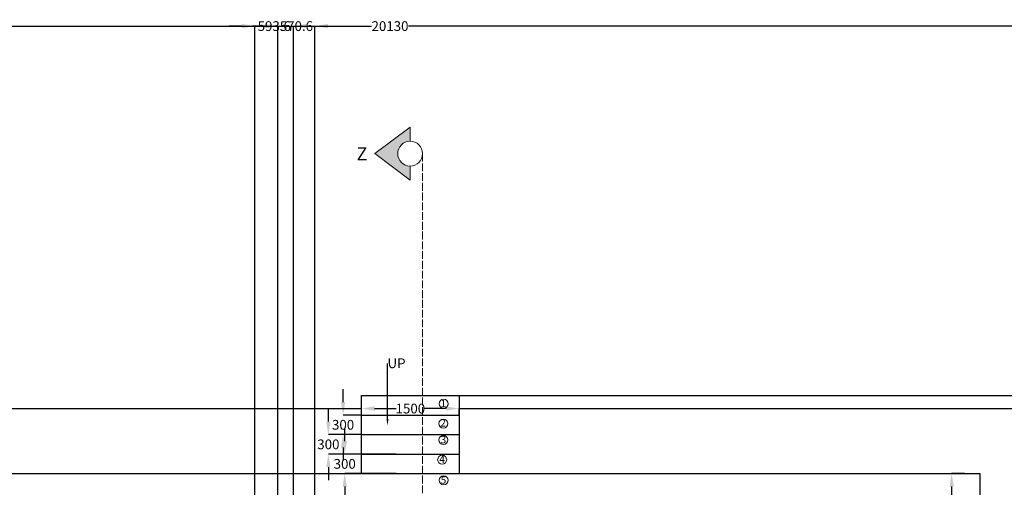
# Model space of a CAD drawing. Units: inches. Extents: x 22626 to 57351, y 2118 to 36234.
# Tile 9 of 10: x 34432 to 49561, y 29046 to 36234. Entities that reach past the tile are written whole.
import ezdxf
from ezdxf import colors
from ezdxf.entities.mleader import LeaderData, LeaderLine
from ezdxf.math import Vec2, Vec3

# ---------------------------------------------------------------- set-up
doc = ezdxf.new("R2010")
doc.units = ezdxf.units.IN
doc.header["$MEASUREMENT"] = 0
doc.linetypes.add('ACAD_ISO02W100', pattern=[15, 12, -3])
for name, color, linetype, lineweight in [('A-ANNO-DIMS', 130, 'Continuous', 18), ('A-ANNO-STRS', 130, 'Continuous', 15), ('A-ANNO-SYMB', 130, 'Continuous', 18), ('A-FLOR', 80, 'Continuous', 30), ('A-ROOF', 80, 'Continuous', 25), ('STAIRS', 82, 'Continuous', 25)]:
    doc.layers.add(name, color=color, linetype=linetype, lineweight=lineweight)
doc.layers.add('A-SECT', color=2, linetype='ACAD_ISO02W100', lineweight=18, true_color=0xf1eb1f)
doc.styles.get("Standard").update_dxf_attribs({"font": 'arial.ttf'})
doc.dimstyles.get("Standard").update_dxf_attribs({"dimtxt": 150, "dimasz": 200, "dimexe": 0.18, "dimexo": 0.0625, "dimgap": 0.09, "dimtad": 0, "dimtih": 1, "dimtoh": 1, "dimdec": 0, "dimzin": 0, "dimdsep": 46, "dimtxsty": 'Standard', "dimcen": 0.09, "dimadec": 0, "dimazin": 0, "dimtfac": 1, "dimtdec": 0, "dimtofl": 0, "dimtmove": 0, "dimatfit": 3, "dimfxl": 1, "dimtolj": 1, "dimtzin": 0, "dimarcsym": 0})

# ---------------------------------------------------------------- blocks, each defined once
blk = doc.blocks.new('*D20')
at = {"layer": 'A-ANNO-DIMS', "color": 0, "lineweight": -2, "transparency": 16777216}
for p, q in [((39426, 29757), (39426, 29957)), ((40218, 29557), (39426, 29557)), ((40218, 29257), (39426, 29257)), ((39426, 29057), (39426, 28857))]:
    blk.add_line(p, q, dxfattribs=at)
at = {"layer": 'A-ANNO-DIMS', "color": 0, "transparency": 16777216}
for points in [[(39393, 29757), (39460, 29757), (39426, 29557)], [(39393, 29057), (39460, 29057), (39426, 29257)]]:
    blk.add_solid(points, dxfattribs=at)
at = {"layer": 'Defpoints', "color": 0, "transparency": 16777216}
for p in [(39426, 29557), (40218, 29557), (40218, 29257)]:
    blk.add_point(p, dxfattribs=at)
at = {"layer": 'A-ANNO-DIMS', "color": 0, "transparency": 16777216, "insert": (39426, 29407), "char_height": 150, "attachment_point": 5}
blk.add_mtext('\\A1;300', dxfattribs=at)
blk = doc.blocks.new('*D21')
at = {"layer": 'A-ANNO-DIMS', "color": 0, "lineweight": -2, "transparency": 16777216}
for p, q in [((39175, 30057), (39175, 30257)), ((39684, 29857), (39175, 29857)), ((39684, 29557), (39175, 29557)), ((39175, 29357), (39175, 29157))]:
    blk.add_line(p, q, dxfattribs=at)
at = {"layer": 'A-ANNO-DIMS', "color": 0, "transparency": 16777216}
for points in [[(39142, 30057), (39208, 30057), (39175, 29857)], [(39142, 29357), (39208, 29357), (39175, 29557)]]:
    blk.add_solid(points, dxfattribs=at)
at = {"layer": 'Defpoints', "color": 0, "transparency": 16777216}
for p in [(39175, 29857), (39685, 29857), (39685, 29557)]:
    blk.add_point(p, dxfattribs=at)
at = {"layer": 'A-ANNO-DIMS', "color": 0, "transparency": 16777216, "insert": (39175, 29707), "char_height": 150, "attachment_point": 5}
blk.add_mtext('\\A1;300', dxfattribs=at)
blk = doc.blocks.new('*D22')
at = {"layer": 'A-ANNO-DIMS', "color": 0, "lineweight": -2, "transparency": 16777216}
for p, q in [((39401, 30357), (39401, 30557)), ((39684, 30157), (39401, 30157)), ((39684, 29857), (39401, 29857)), ((39401, 29657), (39401, 29457))]:
    blk.add_line(p, q, dxfattribs=at)
at = {"layer": 'A-ANNO-DIMS', "color": 0, "transparency": 16777216}
for points in [[(39368, 30357), (39435, 30357), (39401, 30157)], [(39368, 29657), (39435, 29657), (39401, 29857)]]:
    blk.add_solid(points, dxfattribs=at)
at = {"layer": 'Defpoints', "color": 0, "transparency": 16777216}
for p in [(39401, 30157), (39685, 30157), (39685, 29857)]:
    blk.add_point(p, dxfattribs=at)
at = {"layer": 'A-ANNO-DIMS', "color": 0, "transparency": 16777216, "insert": (39401, 30007), "char_height": 150, "attachment_point": 5}
blk.add_mtext('\\A1;300', dxfattribs=at)
blk = doc.blocks.new('*D23')
at = {"layer": 'A-ANNO-DIMS', "color": 0, "lineweight": -2, "transparency": 16777216}
for p, q in [((39685, 30157), (39685, 30257)), ((39885, 30257), (40218, 30257)), ((40985, 30257), (40651, 30257)), ((41185, 30157), (41185, 30257))]:
    blk.add_line(p, q, dxfattribs=at)
at = {"layer": 'A-ANNO-DIMS', "color": 0, "transparency": 16777216}
for points in [[(39885, 30290), (39885, 30224), (39685, 30257)], [(40985, 30290), (40985, 30224), (41185, 30257)]]:
    blk.add_solid(points, dxfattribs=at)
at = {"layer": 'Defpoints', "color": 0, "transparency": 16777216}
for p in [(39685, 30157), (41185, 30257), (41185, 30157)]:
    blk.add_point(p, dxfattribs=at)
at = {"layer": 'A-ANNO-DIMS', "color": 0, "transparency": 16777216, "insert": (40435, 30257), "char_height": 150, "attachment_point": 5}
blk.add_mtext('\\A1;1500', dxfattribs=at)
blk = doc.blocks.new('*D24')
at = {"layer": 'A-ANNO-DIMS', "color": 0, "lineweight": -2, "transparency": 16777216}
for p, q in [((48951, 29257), (48752, 29257)), ((48752, 29057), (48752, 28834)), ((48752, 28457), (48752, 28680)), ((48951, 28257), (48752, 28257))]:
    blk.add_line(p, q, dxfattribs=at)
at = {"layer": 'A-ANNO-DIMS', "color": 0, "transparency": 16777216}
for points in [[(48719, 29057), (48786, 29057), (48752, 29257)], [(48719, 28457), (48786, 28457), (48752, 28257)]]:
    blk.add_solid(points, dxfattribs=at)
at = {"layer": 'Defpoints', "color": 0, "transparency": 16777216}
for p in [(48752, 29257), (48951, 29257), (48951, 28257)]:
    blk.add_point(p, dxfattribs=at)
at = {"layer": 'A-ANNO-DIMS', "color": 0, "transparency": 16777216, "insert": (48752, 28757), "char_height": 150, "attachment_point": 5}
blk.add_mtext('\\A1;1000', dxfattribs=at)
blk = doc.blocks.new('SECTION-HEAD')
h = blk.add_hatch(color=256)
h.dxf.hatch_style = 1
h.paths.add_polyline_path([(815, 541), (599, 541, -1), (216, 541), (0, 541), (407, 0)])
for p, q in [((216, 541), (0, 541)), ((0, 541), (407, 0)), ((815, 541), (407, 0)), ((599, 541), (815, 541))]:
    blk.add_line(p, q)
blk.add_circle((407, 541), 191)
blk = doc.blocks.new('*D98')
at = {"layer": 'A-ANNO-DIMS', "color": 0, "lineweight": -2, "transparency": 16777216}
for p, q in [((30057, 30257), (30057, 36136)), ((30257, 36136), (39839, 36136)), ((49987, 36136), (40406, 36136)), ((50187, 30257), (50187, 36136))]:
    blk.add_line(p, q, dxfattribs=at)
at = {"layer": 'A-ANNO-DIMS', "color": 0, "transparency": 16777216}
for points in [[(30257, 36169), (30257, 36103), (30057, 36136)], [(49987, 36169), (49987, 36103), (50187, 36136)]]:
    blk.add_solid(points, dxfattribs=at)
at = {"layer": 'Defpoints', "color": 0, "transparency": 16777216}
for p in [(50187, 36136), (30057, 30257), (50187, 30257)]:
    blk.add_point(p, dxfattribs=at)
at = {"layer": 'A-ANNO-DIMS', "color": 0, "transparency": 16777216, "insert": (40122, 36136), "char_height": 150, "attachment_point": 5}
blk.add_mtext('\\A1;20130', dxfattribs=at)
blk = doc.blocks.new('*D99')
at = {"layer": 'A-ANNO-DIMS', "color": 0, "lineweight": -2, "transparency": 16777216}
for p, q in [((41185, 30457), (57039, 30457)), ((57039, 30257), (57039, 18934)), ((57039, 7457), (57039, 18780)), ((43702, 7257), (57039, 7257))]:
    blk.add_line(p, q, dxfattribs=at)
at = {"layer": 'A-ANNO-DIMS', "color": 0, "transparency": 16777216}
for points in [[(57005, 30257), (57072, 30257), (57039, 30457)], [(57005, 7457), (57072, 7457), (57039, 7257)]]:
    blk.add_solid(points, dxfattribs=at)
at = {"layer": 'Defpoints', "color": 0, "transparency": 16777216}
for p in [(41185, 30457), (57039, 30457), (43702, 7257)]:
    blk.add_point(p, dxfattribs=at)
at = {"layer": 'A-ANNO-DIMS', "color": 0, "transparency": 16777216, "insert": (57039, 18857), "char_height": 150, "attachment_point": 5}
blk.add_mtext('\\A1;23200', dxfattribs=at)
blk = doc.blocks.new('*D106')
at = {"layer": 'A-ANNO-DIMS', "color": 0, "lineweight": -2, "transparency": 16777216}
for p, q in [((38198, 36136), (37998, 36136)), ((38398, 21952), (38398, 36136)), ((38969, 21952), (38969, 36136)), ((39169, 36136), (39369, 36136))]:
    blk.add_line(p, q, dxfattribs=at)
at = {"layer": 'A-ANNO-DIMS', "color": 0, "transparency": 16777216}
for points in [[(38198, 36169), (38198, 36103), (38398, 36136)], [(39169, 36169), (39169, 36103), (38969, 36136)]]:
    blk.add_solid(points, dxfattribs=at)
at = {"layer": 'Defpoints', "color": 0, "transparency": 16777216}
for p in [(38969, 36136), (38398, 21952), (38969, 21952)]:
    blk.add_point(p, dxfattribs=at)
at = {"layer": 'A-ANNO-DIMS', "color": 0, "transparency": 16777216, "insert": (38684, 36136), "char_height": 150, "attachment_point": 5}
blk.add_mtext('\\A1;570.6', dxfattribs=at)
blk = doc.blocks.new('*D108')
at = {"layer": 'A-ANNO-DIMS', "color": 0, "lineweight": -2, "transparency": 16777216}
for p, q in [((37847, 36136), (37647, 36136)), ((38047, 24856), (38047, 36136)), ((38641, 24856), (38641, 36136)), ((38841, 36136), (39041, 36136))]:
    blk.add_line(p, q, dxfattribs=at)
at = {"layer": 'A-ANNO-DIMS', "color": 0, "transparency": 16777216}
for points in [[(37847, 36169), (37847, 36103), (38047, 36136)], [(38841, 36169), (38841, 36103), (38641, 36136)]]:
    blk.add_solid(points, dxfattribs=at)
at = {"layer": 'Defpoints', "color": 0, "transparency": 16777216}
for p in [(38641, 36136), (38047, 24856), (38641, 24856)]:
    blk.add_point(p, dxfattribs=at)
at = {"layer": 'A-ANNO-DIMS', "color": 0, "transparency": 16777216, "insert": (38344, 36136), "char_height": 150, "attachment_point": 5}
blk.add_mtext('\\A1;593.6', dxfattribs=at)

msp = doc.modelspace()

# ---------------------------------------------------------------- linework, layer by layer
at = {"layer": 'A-ANNO-STRS'}
for centre in [(40946.5, 30330.65), (40940.93, 30026.37), (40943.28, 29775.32), (40923.6, 29469.73), (40946.5, 29155.17)]:
    msp.add_circle(centre, 69.29, dxfattribs=at)
at = {"layer": 'A-FLOR'}
for p, q in [((31057.43, 29256.86), (49187.43, 29256.86)), ((49187.43, 29256.86), (49187.43, 27806.86))]:
    msp.add_line(p, q, dxfattribs=at)
at = {"layer": 'A-ROOF'}
for points in [[(43702.43, 11956.86), (43702.43, 7256.86), (37542.43, 7256.86), (37542.43, 11956.86), (32562.43, 11956.86), (32562.43, 22296.86), (30057.43, 22296.86), (30057.43, 24356.86), (30057.43, 30256.86), (39684.53, 30256.86)], [(41184.53, 30256.86), (50187.43, 30256.86), (50187.43, 25126.86), (50187.43, 22296.86), (48682.43, 22296.86), (48682.43, 11956.86), (43702.43, 11956.86)]]:
    msp.add_lwpolyline(points, dxfattribs=at)
at = {"layer": 'A-SECT', "ltscale": 10}
msp.add_line((40622.43, 34176.08), (40622.43, 4176.35), dxfattribs=at)
at = {"layer": 'STAIRS'}
for p, q in [((39684.53, 29256.86), (39684.53, 30456.86)), ((39684.53, 30456.86), (41184.53, 30456.86)), ((41184.53, 30456.86), (41184.53, 29256.86)), ((39684.53, 30156.86), (41184.53, 30156.86)), ((39684.53, 29856.86), (41184.53, 29856.86)), ((39684.53, 29556.86), (41184.53, 29556.86))]:
    msp.add_line(p, q, dxfattribs=at)

# ---------------------------------------------------------------- block references
at = {"layer": 'A-ANNO-SYMB', "extrusion": (0, 0, -1), "zscale": -1, "rotation": 90}
msp.add_blockref('SECTION-HEAD', (-39890.15, 33768.59), dxfattribs=at)

# ---------------------------------------------------------------- texts
at = {"layer": 'A-ANNO-STRS'}
for s, p in [('1', (40900.37, 30278.95)), ('2', (40894.56, 29980.84)), ('3', (40900.62, 29722.95)), ('4', (40880.34, 29422.65)), ('5', (40901.47, 29102.5))]:
    msp.add_text(s, height=111.39, dxfattribs=at).set_placement(p)
at = {"layer": 'A-ANNO-SYMB'}
msp.add_text('Z', height=200, dxfattribs=at).set_placement((39609.32, 34073.64))

# ---------------------------------------------------------------- dimensions: what is measured, and where the dimension line sits
at = {"layer": 'A-ANNO-DIMS'}
for base, p1, p2, override, picture, middle in [((50187.43, 36136.06), (30057.43, 30256.86), (50187.43, 30256.86), {"dimdec": 0, "dimlfac": 1, "dimrnd": 0, "dimzin": 0, "dimdsep": 46, "dimlunit": 2}, '*D98', (40122.43, 36136.06)), ((38641.03, 36136.06), (38047.43, 24856.11), (38641.03, 24856.11), {"dimdec": 1, "dimlfac": 1, "dimrnd": 0, "dimzin": 0, "dimdsep": 46, "dimlunit": 2}, '*D108', (38344.23, 36136.06)), ((38968.9273, 36136.0593), (38398.2788, 21952.0585), (38968.9273, 21952.0585), {"dimdec": 1, "dimlfac": 1, "dimrnd": 0, "dimzin": 0, "dimdsep": 46, "dimlunit": 2}, '*D106', (38683.603, 36136.0593)), ((41184.53, 30256.86), (39684.53, 30156.86), (41184.53, 30156.86), {"dimclrd": 0, "dimclre": 0, "dimclrt": 0}, '*D23', (40434.53, 30256.86))]:
    dim = msp.add_linear_dim(base=base, p1=p1, p2=p2, dimstyle='Standard', override=override, dxfattribs=at)
    dim.commit()
    dim.dimension.update_dxf_attribs({"geometry": picture, "text_midpoint": middle})
for base, p1, p2, override, picture, middle in [((39401.32, 30156.86), (39684.53, 29856.86), (39684.53, 30156.86), {"dimclrd": 0, "dimclre": 0, "dimclrt": 0}, '*D22', (39401.32, 30006.86)), ((57038.61, 30456.86), (43702.43, 7256.86), (41184.53, 30456.86), {"dimdec": 0, "dimlfac": 1, "dimrnd": 0, "dimzin": 0, "dimdsep": 46, "dimlunit": 2}, '*D99', (57038.61, 18856.86)), ((39175.16, 29856.86), (39684.53, 29556.86), (39684.53, 29856.86), {"dimclrd": 0, "dimclre": 0, "dimclrt": 0}, '*D21', (39175.16, 29706.86)), ((48752.17, 29256.86), (48950.76, 28256.86), (48950.76, 29256.86), {"dimclrd": 0, "dimclre": 0, "dimclrt": 0}, '*D24', (48752.17, 28756.86))]:
    dim = msp.add_linear_dim(base=base, p1=p1, p2=p2, angle=90, dimstyle='Standard', override=override, dxfattribs=at)
    dim.commit()
    dim.dimension.update_dxf_attribs({"geometry": picture, "text_midpoint": middle})
dim = msp.add_linear_dim(base=(39426.18, 29556.86), p1=(40218.02, 29256.86), p2=(40218.02, 29556.86), angle=90, dimstyle='Standard', override={"dimclrd": 0, "dimclre": 0, "dimclrt": 0}, dxfattribs=at)
dim.commit()
dim.dimension.update_dxf_attribs({"geometry": '*D20', "text_midpoint": (39426.18, 29406.86), "dimtype": 160})

# ---------------------------------------------------------------- leaders
at = {"layer": 'A-ANNO-STRS'}
ml = msp.add_multileader_mtext('Standard', dxfattribs=at)
ml.set_content('UP ', color=256)
ml.set_leader_properties()
ml.build(insert=Vec2(0, 0))
ml.multileader.update_dxf_attribs({"dogleg_length": 0.36, "arrow_head_size": 100})
ctx = ml.context
ctx.base_point, ctx.char_height, ctx.arrow_head_size, ctx.landing_gap_size, ctx.plane_origin = Vec3(40083.82, 30951.92), 150, 100, 0.09, Vec3(40083.46, 29998.93)
notes = []
notes.append((ctx, [(0, (1, 1, 0), (40083.46, 30951.92), (1, 0), 0.36, [(0, [(40083.46, 29998.93), (40083.46, 30947.38), (40083.46, 30951.92)], 0, [])])]))
ctx.mtext.insert, ctx.mtext.flow_direction = Vec3(40083.91, 31028.2), 5
for ctx, leaders in notes:
    for number, flags, end, landing, length, lines in leaders:
        leader = LeaderData()
        leader.index, (leader.has_last_leader_line, leader.has_dogleg_vector, leader.attachment_direction) = number, flags
        leader.last_leader_point, leader.dogleg_vector, leader.dogleg_length = Vec3(end), Vec3(landing), length
        for number, points, colour, breaks in lines:
            line = LeaderLine()
            line.index, line.vertices, line.color, line.breaks = number, Vec3.list(points), colors.encode_raw_color(colour), breaks
            leader.lines.append(line)
        ctx.leaders.append(leader)

doc.saveas('drawing.dxf')
